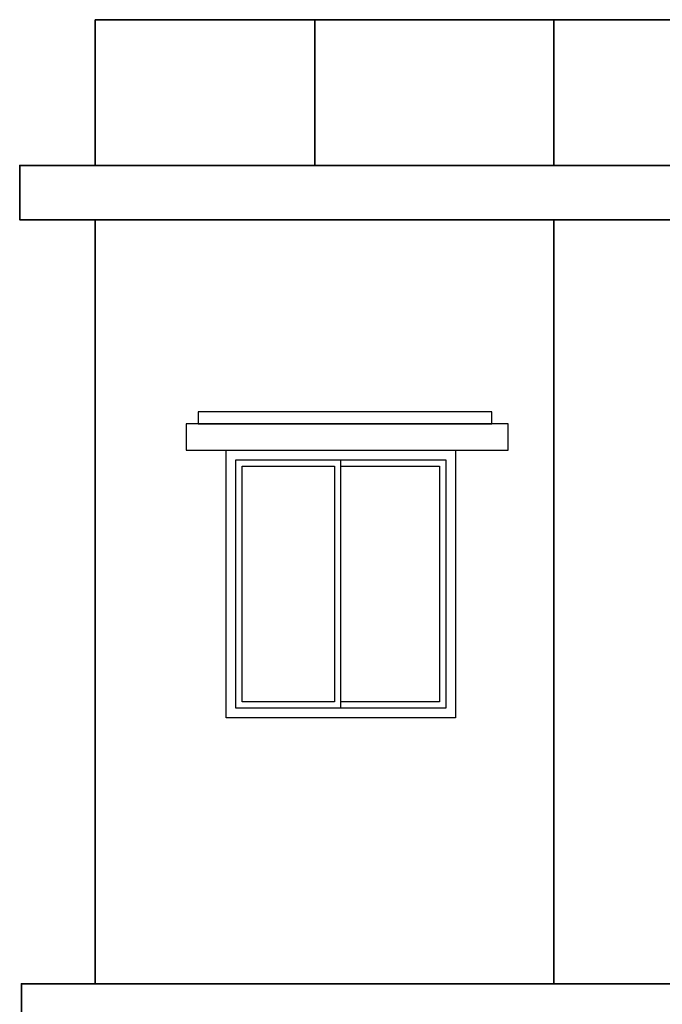
# Model space of a CAD drawing. Units: inches. Extents: x 3 to 303, y 4 to 326.
# Tile 4 of 6: x 3 to 104, y 120 to 275. Entities that reach past the tile are written whole.
import ezdxf

# ---------------------------------------------------------------- set-up
doc = ezdxf.new("R2010")
doc.units = ezdxf.units.IN
doc.header["$MEASUREMENT"] = 0
doc.layers.add('A-ELEV', color=7, linetype='Continuous', lineweight=35)
doc.layers.add('A-GLAZ', color=4, linetype='Continuous', lineweight=25)

# ---------------------------------------------------------------- blocks, each defined once
blk = doc.blocks.new('*U2')
for p, q in [((1.5, 1.5), (1.5, 40.5)), ((1.5, 40.5), (18, 40.5)), ((18, 1.5), (18, 40.5)), ((18, 40.5), (34.5, 40.5)), ((34.5, 40.5), (34.5, 1.5)), ((18, 1.5), (1.5, 1.5)), ((34.5, 1.5), (18, 1.5))]:
    blk.add_line(p, q)
blk.add_lwpolyline([(0, 0), (0, 42), (36, 42), (36, 0)], close=True)
for points in [[(17, 39.5), (17, 2.5), (2.5, 2.5), (2.5, 39.5), (17, 39.5)], [(18, 39.5), (33.5, 39.5), (33.5, 2.5), (18, 2.5)]]:
    blk.add_lwpolyline(points)

msp = doc.modelspace()

# ---------------------------------------------------------------- linework, layer by layer
at = {"layer": 'A-ELEV'}
for p, q in [((87.23, 275.03), (15.23, 275.03)), ((15.23, 275.03), (15.23, 252.13)), ((49.71, 252.13), (49.71, 275.03)), ((178.79, 275.03), (87.23, 275.03)), ((87.23, 275.03), (87.23, 252.13)), ((164.01, 252.13), (15.23, 252.13)), ((219.23, 243.62), (15.23, 243.62)), ((15.23, 243.62), (15.23, 123.62)), ((87.23, 243.62), (49.71, 243.62)), ((87.23, 243.62), (87.23, 123.62)), ((219.23, 123.62), (15.23, 123.62)), ((15.23, 123.62), (219.23, 123.62))]:
    msp.add_line(p, q, dxfattribs=at)
for points in [[(15.23, 243.62), (3.37, 243.62), (3.37, 252.13), (15.23, 252.13)], [(15.23, 111.62), (3.64, 111.62), (3.64, 123.62), (15.23, 123.62)]]:
    msp.add_lwpolyline(points, dxfattribs=at)
at = {"layer": 'A-GLAZ'}
for points in [[(31.41, 211.56), (77.5, 211.56), (77.5, 213.44), (31.41, 213.44)], [(29.53, 207.41), (80.06, 207.41), (80.06, 211.56), (29.53, 211.56)]]:
    msp.add_lwpolyline(points, close=True, dxfattribs=at)

# ---------------------------------------------------------------- block references
msp.add_blockref('*U2', (35.8, 165.41), dxfattribs=at)

doc.saveas('drawing.dxf')
